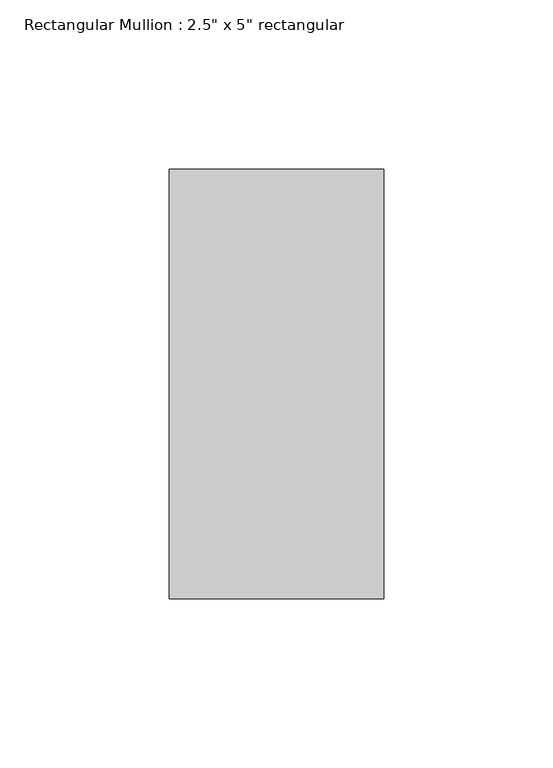
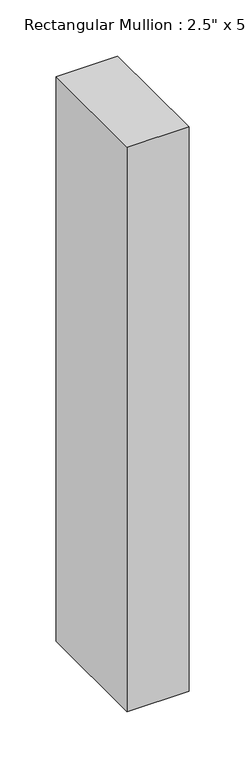
"""IFC4 building model written with IfcOpenShell, lengths in millimetres: member geometry."""

from ifc_helpers import new_model, si_unit, frame, origin, place, context, project, spatial, polyline, outline, extrude, source, transform, mapped, element, save


def member_67fa2ece(model_context):
    return source(origin(), model_context, "Body", "SweptSolid", [
        extrude(outline(polyline([(0.0, 63.5), (0.0, -63.5), (-63.5, -63.5), (-63.5, 63.5), (0.0, 63.5)])), frame((0.0, 0.0, -613.7328955), z_axis=(0.0, 0.0, 1.0), x_axis=(1.0, 0.0, 0.0)), (0.0, 0.0, 1.0), 613.7328955),
    ])


if __name__ == "__main__":
    model = new_model("IFC4")
    model_context = context("Model", 3, world=origin())
    ifc_project = project(units=[si_unit("LENGTHUNIT", "METRE", prefix="MILLI")], contexts=[model_context])
    site = spatial("IfcSite", under=ifc_project)
    building = spatial("IfcBuilding", under=site)
    placement = place(None, origin())
    member_shape = member_67fa2ece(model_context)
    element("IfcMember", 1, ObjectType="Rectangular Mullion : 2.5\" x 5\" rectangular", at=placement, inside=building, context=model_context, shape_type="MappedRepresentation", body=[
        mapped(member_shape, transform((0.0, 0.0, 0.0), x_axis=(1.0, 0.0, 0.0), y_axis=(0.0, 1.0, 0.0), z_axis=(0.0, 0.0, 1.0))),
    ])
    save(model, "model.ifc")

# Revit data of these elements
# Type "Rectangular Mullion : 2.5\" x 5\" rectangular"
#   built-in parameter 1007304 = 0.416667 (stored number, unit not read)
#   built-in parameter 1007301 = 0.104167 (stored number, unit not read)
#   built-in parameter 1007300 = 0.104167 (stored number, unit not read)
# Element 1 (IfcMember, "Rectangular Mullion : 2.5\" x 5\" rectangular")
#   Materials on its faces: "Aluminum"
# Materials
#   "Aluminum": class "Metal", colour RGB 247 247 247, transparency 0, Description = "Aluminum 6061", Cost = 0
